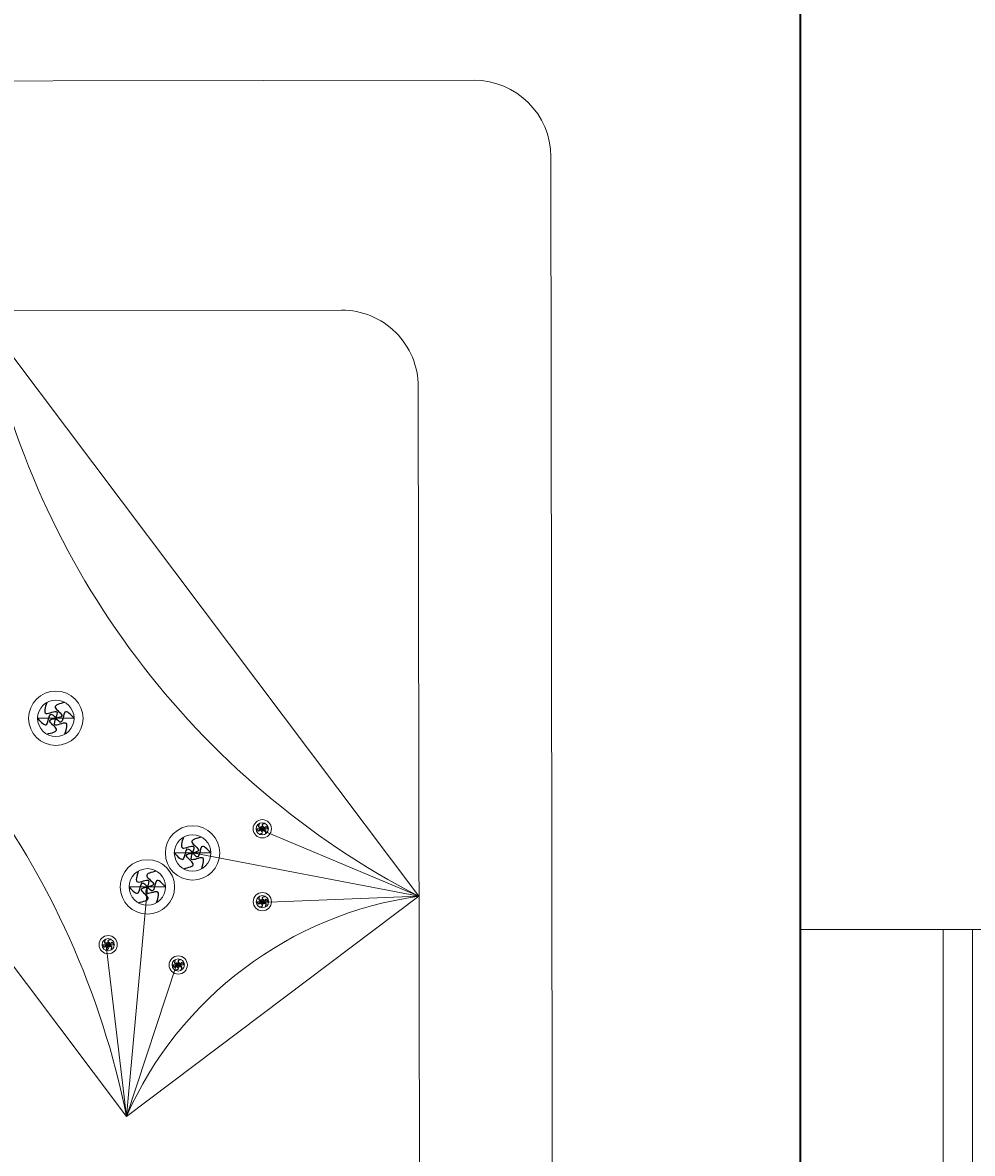
# Model space of a CAD drawing. Units: inches. Extents: x -61 to 1599, y -1316 to 257.
# Tile 139 of 204: x 515 to 540, y -104 to -74. Entities that reach past the tile are written whole.
import ezdxf

# ---------------------------------------------------------------- set-up
doc = ezdxf.new("R2010")
doc.units = ezdxf.units.IN
doc.header["$MEASUREMENT"] = 0
for name, color, linetype, lineweight in [('A-ANNO-DIMS', 2, 'Continuous', 18), ('FURNITURE', 83, 'Continuous', 18), ('WALLS', 4, 'Continuous', 35), ('WINDOWS', 220, 'Continuous', 18)]:
    doc.layers.add(name, color=color, linetype=linetype, lineweight=lineweight)
doc.layers.add('FUR', color=83, linetype='Continuous')
doc.styles.get("Standard").update_dxf_attribs({"font": 'arial.ttf'})
doc.dimstyles.get("Standard").update_dxf_attribs({"dimtxt": 0.18, "dimasz": 0.18, "dimexe": 0.18, "dimexo": 0.0625, "dimgap": 0.09, "dimtad": 0, "dimtih": 1, "dimtoh": 1, "dimdec": 0, "dimzin": 0, "dimdsep": 46, "dimlunit": 3, "dimtxsty": 'Standard', "dimcen": 0.09, "dimadec": 0, "dimazin": 0, "dimtfac": 1, "dimtdec": 0, "dimtofl": 0, "dimtmove": 0, "dimatfit": 3, "dimfxl": 1, "dimtolj": 1, "dimtzin": 0, "dimarcsym": 0})

# ---------------------------------------------------------------- blocks, each defined once
blk = doc.blocks.new('*U215')
at = {"layer": 'FUR'}
blk.add_open_spline([(0.015, 0.238), (-0.088, 0.143), (-0.292, -0.045), (0.224, -0.053), (0.072, -0.187), (0.015, -0.238)], degree=3, knots=[0, 0, 0, 0, 0.2846533, 0.5662105, 0.736751, 0.736751, 0.736751, 0.736751], dxfattribs=at)
blk = doc.blocks.new('*U216')
at = {"layer": 'FURNITURE', "transparency": 16777216}
for p, rotation in [((662.517, -238.489), 60), ((662.929, -238.463), 300), ((662.531, -238.727), 120), ((662.745, -238.833), 180), ((662.944, -238.702), 240)]:
    blk.add_blockref('*U215', p, dxfattribs=dict(at, rotation=rotation))
blk.add_blockref('*U215', (662.716, -238.357), dxfattribs=at)
blk = doc.blocks.new('*U252')
at = {"layer": 'FUR'}
blk.add_open_spline([(0.015, 0.238), (-0.088, 0.143), (-0.292, -0.045), (0.224, -0.053), (0.072, -0.187), (0.015, -0.238)], degree=3, knots=[0, 0, 0, 0, 0.2846533, 0.5662105, 0.736751, 0.736751, 0.736751, 0.736751], dxfattribs=at)
blk = doc.blocks.new('*U234')
at = {"layer": 'FURNITURE', "transparency": 16777216}
for p, rotation in [((662.517, -238.489), 60), ((662.929, -238.463), 300), ((662.531, -238.727), 120), ((662.745, -238.833), 180), ((662.944, -238.702), 240)]:
    blk.add_blockref('*U252', p, dxfattribs=dict(at, rotation=rotation))
blk.add_blockref('*U252', (662.716, -238.357), dxfattribs=at)
blk = doc.blocks.new('*U235')
at = {"layer": 'FUR'}
blk.add_open_spline([(0.005, 0.08), (-0.03, 0.048), (-0.098, -0.015), (0.075, -0.018), (0.024, -0.063), (0.005, -0.08)], degree=3, knots=[0, 0, 0, 0, 0.0954578, 0.1898773, 0.2470677, 0.2470677, 0.2470677, 0.2470677], dxfattribs=at)
blk = doc.blocks.new('*U236')
at = {"layer": 'FURNITURE', "transparency": 16777216}
for p, rotation in [((222.173, -79.977), 60), ((222.178, -80.056), 120), ((222.25, -80.092), 180), ((222.312, -79.968), 300), ((222.317, -80.048), 240)]:
    blk.add_blockref('*U235', p, dxfattribs=dict(at, rotation=rotation))
blk.add_blockref('*U235', (222.24, -79.932), dxfattribs=at)
blk = doc.blocks.new('*U217')
at = {"layer": 'FUR'}
blk.add_open_spline([(0.005, 0.08), (-0.03, 0.048), (-0.098, -0.015), (0.075, -0.018), (0.024, -0.063), (0.005, -0.08)], degree=3, knots=[0, 0, 0, 0, 0.0954578, 0.1898773, 0.2470677, 0.2470677, 0.2470677, 0.2470677], dxfattribs=at)
blk = doc.blocks.new('*U241')
at = {"layer": 'FURNITURE', "transparency": 16777216}
for p, rotation in [((222.173, -79.977), 60), ((222.178, -80.056), 120), ((222.25, -80.092), 180), ((222.312, -79.968), 300), ((222.317, -80.048), 240)]:
    blk.add_blockref('*U217', p, dxfattribs=dict(at, rotation=rotation))
blk.add_blockref('*U217', (222.24, -79.932), dxfattribs=at)
blk = doc.blocks.new('*U242')
at = {"layer": 'FUR'}
blk.add_open_spline([(0.005, 0.08), (-0.03, 0.048), (-0.098, -0.015), (0.075, -0.018), (0.024, -0.063), (0.005, -0.08)], degree=3, knots=[0, 0, 0, 0, 0.0954578, 0.1898773, 0.2470677, 0.2470677, 0.2470677, 0.2470677], dxfattribs=at)
blk = doc.blocks.new('*U243')
at = {"layer": 'FURNITURE', "transparency": 16777216}
for p, rotation in [((222.173, -79.977), 60), ((222.178, -80.056), 120), ((222.25, -80.092), 180), ((222.312, -79.968), 300), ((222.317, -80.048), 240)]:
    blk.add_blockref('*U242', p, dxfattribs=dict(at, rotation=rotation))
blk.add_blockref('*U242', (222.24, -79.932), dxfattribs=at)
blk = doc.blocks.new('*U244')
at = {"layer": 'FUR'}
blk.add_open_spline([(0.005, 0.08), (-0.03, 0.048), (-0.098, -0.015), (0.075, -0.018), (0.024, -0.063), (0.005, -0.08)], degree=3, knots=[0, 0, 0, 0, 0.0954578, 0.1898773, 0.2470677, 0.2470677, 0.2470677, 0.2470677], dxfattribs=at)
blk = doc.blocks.new('*U245')
at = {"layer": 'FURNITURE', "transparency": 16777216}
for p, rotation in [((222.173, -79.977), 60), ((222.178, -80.056), 120), ((222.25, -80.092), 180), ((222.312, -79.968), 300), ((222.317, -80.048), 240)]:
    blk.add_blockref('*U244', p, dxfattribs=dict(at, rotation=rotation))
blk.add_blockref('*U244', (222.24, -79.932), dxfattribs=at)
blk = doc.blocks.new('*U213')
at = {"layer": 'FUR'}
blk.add_open_spline([(0.015, 0.238), (-0.088, 0.143), (-0.292, -0.045), (0.224, -0.053), (0.072, -0.187), (0.015, -0.238)], degree=3, knots=[0, 0, 0, 0, 0.2846533, 0.5662105, 0.736751, 0.736751, 0.736751, 0.736751], dxfattribs=at)
blk = doc.blocks.new('*U214')
at = {"layer": 'FURNITURE', "transparency": 16777216}
for p, rotation in [((662.517, -238.489), 60), ((662.929, -238.463), 300), ((662.531, -238.727), 120), ((662.745, -238.833), 180), ((662.944, -238.702), 240)]:
    blk.add_blockref('*U213', p, dxfattribs=dict(at, rotation=rotation))
blk.add_blockref('*U213', (662.716, -238.357), dxfattribs=at)
blk = doc.blocks.new('WIN-36IN')
for p, q in [((36, 9), (36, 0)), ((0, 5.262), (36, 5.262)), ((0, 4.5), (36, 4.5)), ((0, 4.5), (36, 4.5))]:
    blk.add_line(p, q)
blk = doc.blocks.new('*D704')
at = {"layer": 'A-ANNO-DIMS', "color": 0, "lineweight": -2, "transparency": 16777216}
for p, q in [((491.833, -616.882), (491.833, 257.457)), ((492.013, 257.277), (517.874, 257.277)), ((544.523, 257.277), (518.661, 257.277)), ((544.703, -616.882), (544.703, 257.457))]:
    blk.add_line(p, q, dxfattribs=at)
at = {"layer": 'A-ANNO-DIMS', "color": 0, "transparency": 16777216}
for points in [[(492.013, 257.307), (492.013, 257.247), (491.833, 257.277)], [(544.523, 257.307), (544.523, 257.247), (544.703, 257.277)]]:
    blk.add_solid(points, dxfattribs=at)
at = {"layer": 'DEFPOINTS', "color": 0, "transparency": 16777216}
for p in [(544.703, 257.277), (491.833, -616.945), (544.703, -616.945)]:
    blk.add_point(p, dxfattribs=at)
at = {"layer": 'A-ANNO-DIMS', "color": 0, "transparency": 16777216, "insert": (518.268, 257.277), "char_height": 0.18, "attachment_point": 5}
blk.add_mtext('\\A1;52.87', dxfattribs=at)

msp = doc.modelspace()

# ---------------------------------------------------------------- linework, layer by layer
at = {"layer": 'FURNITURE'}
for p, q in [((506.7579, -81.8149), (523.7299, -81.7915)), ((525.7931, -127.7888), (525.7326, -83.7888)), ((516.2688, -92.452), (515.7923, -92.4527)), ((516.2688, -92.452), (516.7452, -92.4514)), ((521.6593, -95.3388), (521.4995, -95.339)), ((525.7509, -97.1025), (521.6068, -95.3582)), ((521.6593, -95.3388), (521.8191, -95.3385)), ((519.8388, -95.9691), (519.3623, -95.9698)), ((519.8388, -95.9691), (520.3153, -95.9685)), ((525.7509, -97.1025), (519.8388, -95.9691)), ((518.1128, -102.851), (518.6602, -96.8562)), ((518.6602, -96.8562), (518.1837, -96.8568)), ((518.6602, -96.8562), (519.1367, -96.8555)), ((525.7509, -97.1025), (521.6094, -97.2623)), ((521.6619, -97.2429), (521.5021, -97.2431)), ((521.6619, -97.2429), (521.8217, -97.2427)), ((517.6362, -98.3665), (517.4764, -98.3667)), ((518.1128, -102.851), (517.5838, -98.386)), ((517.6362, -98.3665), (517.796, -98.3663)), ((518.1128, -102.851), (519.4128, -98.9155)), ((519.4652, -98.8961), (519.3054, -98.8963)), ((519.4652, -98.8961), (519.625, -98.8959))]:
    msp.add_line(p, q, dxfattribs=at)
msp.add_lwpolyline([(503.2659, -129.8197), (503.2714, -133.8197, 0.4142136), (505.2742, -135.817), (527.2741, -135.7867, 0.4142137), (529.2714, -133.784), (529.1944, -77.784, 0.4142134), (527.1916, -75.7868), (505.1917, -75.817, 0.4142136), (503.1944, -77.8197), (503.1999, -81.8197)], format="xyb", dxfattribs=at)
msp.add_lwpolyline([(518.1128, -102.851), (506.7866, -87.8015), (514.4247, -82.0531), (525.7509, -97.1025)], close=True, dxfattribs=at)
for centre, radius in [((516.2688, -92.452), 0.7104), ((516.2688, -92.452), 0.4765), ((521.6593, -95.3388), 0.2382), ((519.8388, -95.9691), 0.7104), ((521.6593, -95.3388), 0.1598), ((519.8388, -95.9691), 0.4765), ((518.6602, -96.8562), 0.7104), ((518.6602, -96.8562), 0.4765), ((521.6619, -97.2429), 0.2382), ((521.6619, -97.2429), 0.1598), ((517.6362, -98.3665), 0.2382), ((517.6362, -98.3665), 0.1598), ((519.4652, -98.8961), 0.2382), ((519.4652, -98.8961), 0.1598)]:
    msp.add_circle(centre, radius, dxfattribs=at)
for centre, radius, start, end in [((523.7326, -83.7915), 2, 0.07875, 90.07876), ((535.7357, -77.8012), 21.731, 191.28318, 242.64711), ((496.8019, -107.1028), 21.731, 11.28318, 62.64711), ((527.0875, -106.8271), 9.816, 97.82577, 156.10452)]:
    msp.add_arc(centre, radius, start, end, dxfattribs=at)
at = {"layer": 'WALLS'}
msp.add_line((535.7028, -13.3229), (535.7028, -175.3229), dxfattribs=at)

# ---------------------------------------------------------------- block references
at = {"layer": 'FURNITURE', "rotation": 270.0787336990067}
for name, p in [('*U216', (753.953, 570.6054)), ('*U236', (601.3661, 127.0159)), ('*U234', (757.5231, 567.0882)), ('*U214', (756.3445, 566.2012)), ('*U241', (601.3687, 125.1118)), ('*U245', (597.343, 123.9882)), ('*U243', (599.1721, 123.4586))]:
    msp.add_blockref(name, p, dxfattribs=at)
at = {"layer": 'WINDOWS', "rotation": 90.00000000000011}
msp.add_blockref('WIN-36IN', (544.7029, -133.972), dxfattribs=at)

# ---------------------------------------------------------------- dimensions: what is measured, and where the dimension line sits
at = {"layer": 'A-ANNO-DIMS'}
dim = msp.add_linear_dim(base=(544.7028, 257.2771), p1=(491.8327, -616.9446), p2=(544.7028, -616.9446), dimstyle='Standard', override={"dimdec": 2, "dimlfac": 1, "dimrnd": 0, "dimzin": 0, "dimdsep": 46, "dimlunit": 2}, dxfattribs=at)
dim.commit()
dim.dimension.update_dxf_attribs({"geometry": '*D704', "text_midpoint": (518.2677, 257.2771)})

doc.saveas('drawing.dxf')
